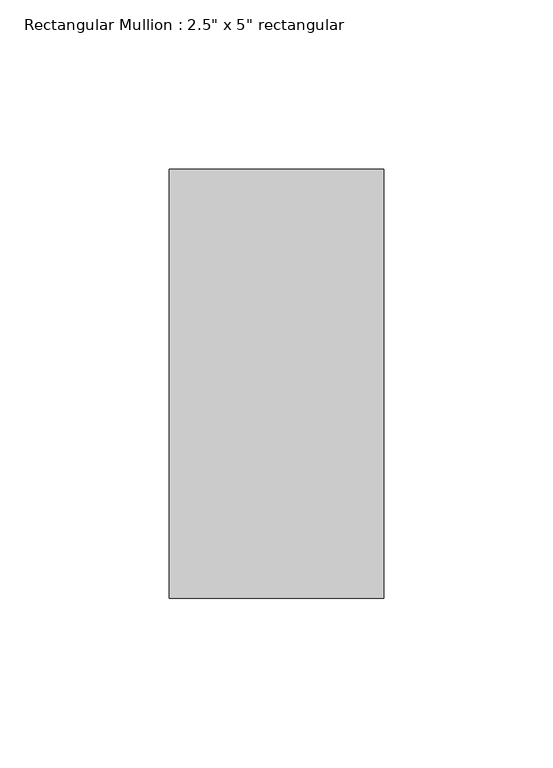
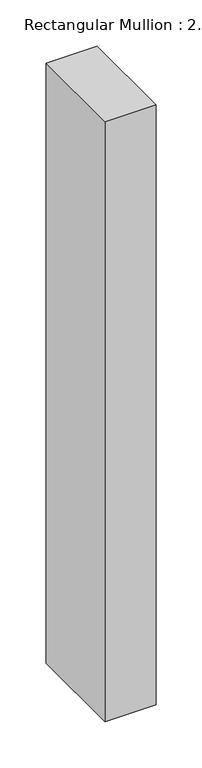
"""IFC4 building model written with IfcOpenShell, lengths in millimetres: member geometry."""

from ifc_helpers import new_model, si_unit, frame, origin, place, context, project, spatial, polyline, outline, extrude, source, transform, mapped, element, save


def member_e59bf7ef(model_context):
    return source(origin(), model_context, "Body", "SweptSolid", [
        extrude(outline(polyline([(31.75, 63.5), (31.75, -63.5), (-31.75, -63.5), (-31.75, 63.5), (31.75, 63.5)])), frame((0.0, 0.0, -791.2941631), z_axis=(0.0, 0.0, 1.0), x_axis=(1.0, 0.0, 0.0)), (0.0, 0.0, 1.0), 791.2941631),
    ])


if __name__ == "__main__":
    model = new_model("IFC4")
    model_context = context("Model", 3, world=origin())
    ifc_project = project(units=[si_unit("LENGTHUNIT", "METRE", prefix="MILLI")], contexts=[model_context])
    site = spatial("IfcSite", under=ifc_project)
    building = spatial("IfcBuilding", under=site)
    placement = place(None, origin())
    member_shape = member_e59bf7ef(model_context)
    element("IfcMember", 1, ObjectType="Rectangular Mullion : 2.5\" x 5\" rectangular", at=placement, inside=building, context=model_context, shape_type="MappedRepresentation", body=[
        mapped(member_shape, transform((0.0, 0.0, 0.0), x_axis=(1.0, 0.0, 0.0), y_axis=(0.0, 1.0, 0.0), z_axis=(0.0, 0.0, 1.0))),
    ])
    save(model, "model.ifc")

# Revit data of these elements
# Type "Rectangular Mullion : 2.5\" x 5\" rectangular"
#   built-in parameter 1007304 = 0.416667 (stored number, unit not read)
#   built-in parameter 1007301 = 0.104167 (stored number, unit not read)
#   built-in parameter 1007300 = 0.104167 (stored number, unit not read)
# Element 1 (IfcMember, "Rectangular Mullion : 2.5\" x 5\" rectangular")
#   Materials on its faces: "Aluminum"
# Materials
#   "Aluminum": class "Metal", colour RGB 247 247 247, transparency 0, Description = "Aluminum 6061", Cost = 0
